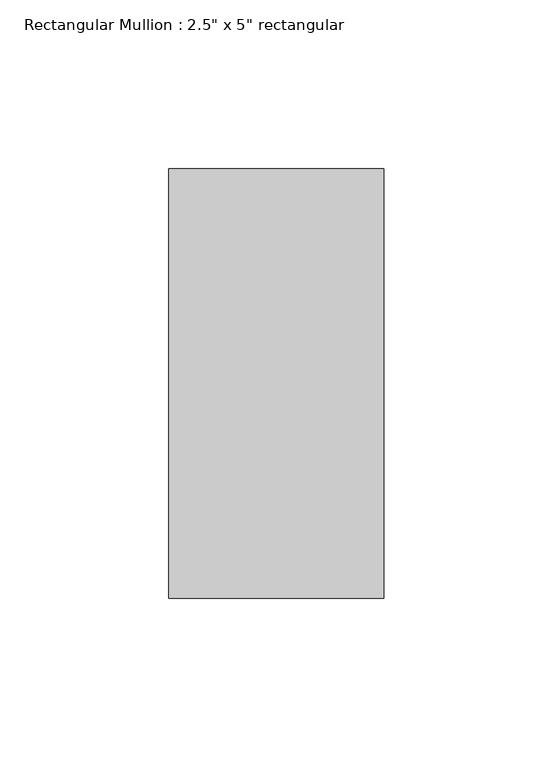
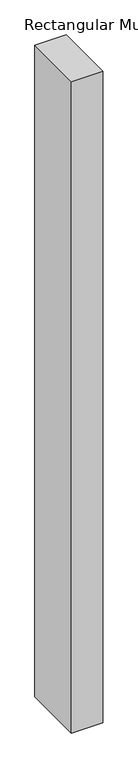
"""IFC4 building model written with IfcOpenShell, lengths in millimetres: member geometry."""

from ifc_helpers import new_model, si_unit, frame, origin, place, context, project, spatial, polyline, outline, extrude, source, transform, mapped, element, save


def member_4dfd3f86(model_context):
    return source(origin(), model_context, "Body", "SweptSolid", [
        extrude(outline(polyline([(31.75, 63.5), (31.75, -63.5), (-31.75, -63.5), (-31.75, 63.5), (31.75, 63.5)])), frame((0.0, 0.0, -1384.7839289), z_axis=(0.0, 0.0, 1.0), x_axis=(1.0, 0.0, 0.0)), (0.0, 0.0, 1.0), 1384.7839289),
    ])


if __name__ == "__main__":
    model = new_model("IFC4")
    model_context = context("Model", 3, world=origin())
    ifc_project = project(units=[si_unit("LENGTHUNIT", "METRE", prefix="MILLI")], contexts=[model_context])
    site = spatial("IfcSite", under=ifc_project)
    building = spatial("IfcBuilding", under=site)
    placement = place(None, origin())
    member_shape = member_4dfd3f86(model_context)
    element("IfcMember", 1, ObjectType="Rectangular Mullion : 2.5\" x 5\" rectangular", at=placement, inside=building, context=model_context, shape_type="MappedRepresentation", body=[
        mapped(member_shape, transform((0.0, 0.0, 0.0), x_axis=(1.0, 0.0, 0.0), y_axis=(0.0, 1.0, 0.0), z_axis=(0.0, 0.0, 1.0))),
    ])
    save(model, "model.ifc")

# Revit data of these elements
# Type "Rectangular Mullion : 2.5\" x 5\" rectangular"
#   built-in parameter 1007304 = 0.416667 (stored number, unit not read)
#   built-in parameter 1007301 = 0.104167 (stored number, unit not read)
#   built-in parameter 1007300 = 0.104167 (stored number, unit not read)
# Element 1 (IfcMember, "Rectangular Mullion : 2.5\" x 5\" rectangular")
#   Materials on its faces: "Aluminum"
# Materials
#   "Aluminum": class "Metal", colour RGB 247 247 247, transparency 0, Description = "Aluminum 6061", Cost = 0
